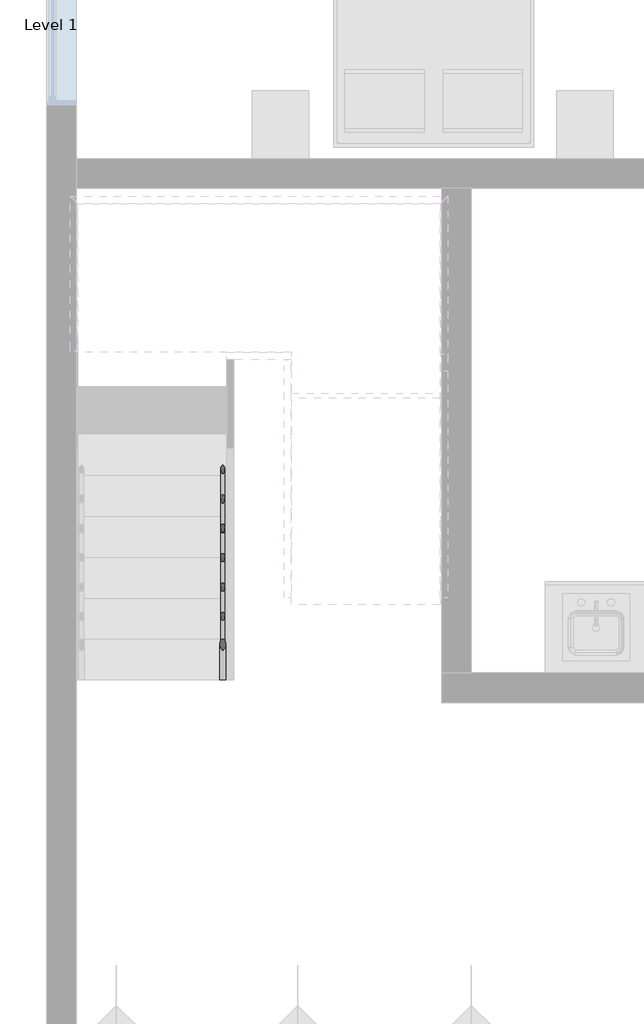
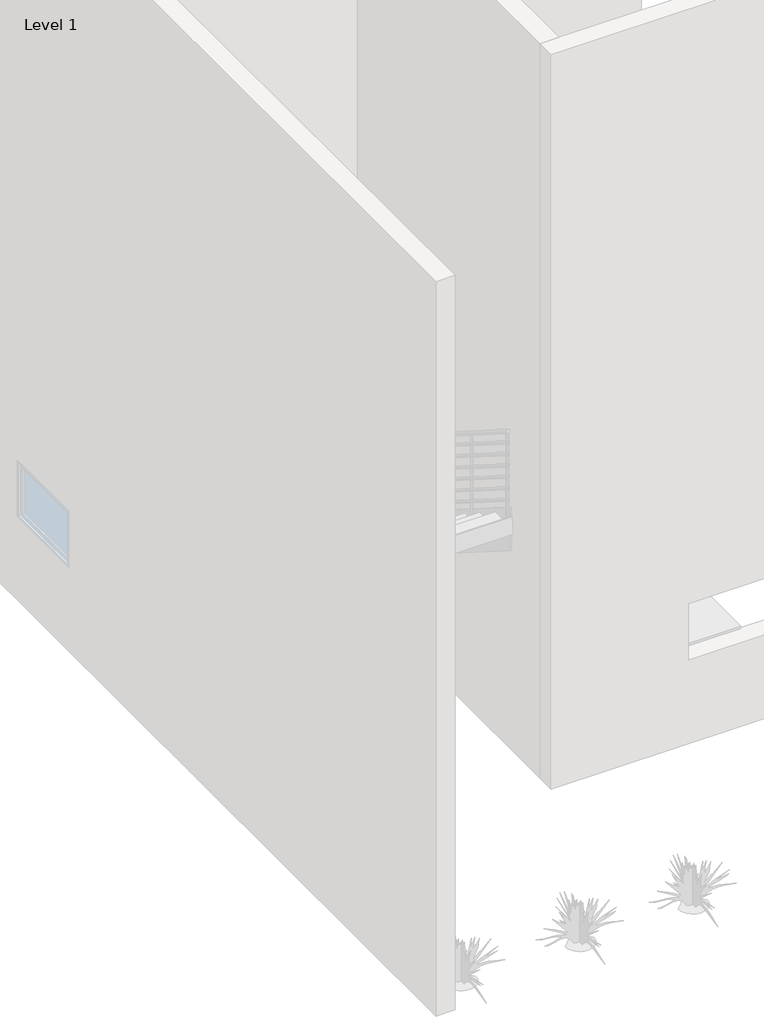
# One storey, part 2 of 4: 1 railing.
"""IFC4 building model written with IfcOpenShell, lengths in millimetres."""

from ifc_helpers import new_model, si_unit, point, frame, frame_2d, origin, place, context, project, spatial, circle_curve, ellipse_curve, trimmed, segment, composite_curve, outline, extrude, element, save
from ifc_brep_helpers import plane_surface, cylinder_surface, advanced_brep

model = new_model("IFC4")

# Units and contexts
model_context = context("Model", 3, world=origin())
ifc_project = project(units=[si_unit("LENGTHUNIT", "METRE", prefix="MILLI")], contexts=[model_context])

# Site, building, storey
site = spatial("IfcSite", under=ifc_project)
building = spatial("IfcBuilding", under=site)
storey = spatial("IfcBuildingStorey", under=building, Name="Level 1", Elevation=0.0)

# Railing
placement = place(None, origin())
element("IfcRailing", 1, ObjectType="900mm Pipe", at=placement, inside=storey, context=model_context, shape_type="SolidModel", body=[
    advanced_brep(
    [(-11027.5547869, 827.4280728, 1050.2491997), (-11067.5547869, 827.4280728, 1050.2491997), (-11027.5547869, 3046.614561, 2453.687295), (-11067.5547869, 3080.4214102, 2475.0671206)],
    [
        (0, 1, ellipse_curve(frame((-11047.5547869, 827.4280728, 1050.2491997), z_axis=(0.0, -1.0, 0.0), x_axis=(0.0, 0.0, -1.0)), 23.6638438, 20.0)),
        (1, 0, ellipse_curve(frame((-11047.5547869, 827.4280728, 1050.2491997), z_axis=(0.0, -1.0, 0.0), x_axis=(0.0, 0.0, -1.0)), 23.6638438, 20.0)),
        (2, 3, ellipse_curve(frame((-11047.5547869, 3063.5179856, 2464.3772078), z_axis=(0.7071067811865486, 0.5976263089853405, 0.37794549184843695), x_axis=(0.7071067811865465, -0.5976263089853425, -0.37794549184843734)), 28.2842712, 20.0)),
        (3, 2, ellipse_curve(frame((-11047.5547869, 3063.5179856, 2464.3772078), z_axis=(0.7071067811865486, 0.5976263089853405, 0.37794549184843695), x_axis=(0.7071067811865465, -0.5976263089853425, -0.37794549184843734)), 28.2842712, 20.0)),
        (0, 2),
        (3, 1),
    ],
    [
        plane_surface(frame((-11047.5547869, 827.4280728, 1073.9130435), z_axis=(0.0, -1.0, 0.0), x_axis=(0.0, 0.0, 1.0))),
        plane_surface(frame((-11047.5547869, 3052.8280728, 2481.2806324), z_axis=(0.7071067811865486, 0.5976263089853405, 0.37794549184843695), x_axis=(0.7071067811865466, -0.5976263089853422, -0.377945491848438))),
        cylinder_surface(frame((-11047.5547869, 838.1179856, 1057.0096189), z_axis=(0.0, -0.845171231398044, -0.5344956404098299), x_axis=(-1.0, 0.0, 0.0)), 20.0),
    ],
    [
        (0, [[1, 2]]),
        (1, [[3, 4]]),
        (2, [[-1, 5, -4, 6]]),
        (2, [[-2, -6, -3, -5]]),
    ],
),
    advanced_brep(
    [(-11019.9614494, 3032.8280728, 2445.2173913), (-11053.7682987, 3072.8280728, 2445.2173913), (-10566.3940799, 3032.8280728, 2445.2173913), (-10532.5872307, 3072.8280728, 2445.2173913)],
    [
        (0, 1, ellipse_curve(frame((-11036.8648741, 3052.8280728, 2445.2173913), z_axis=(-0.7071067811865486, -0.5976263089853405, -0.37794549184843695), x_axis=(-0.7071067811865466, 0.5976263089853426, 0.37794549184843723)), 28.2842712, 20.0)),
        (1, 0, ellipse_curve(frame((-11036.8648741, 3052.8280728, 2445.2173913), z_axis=(-0.7071067811865486, -0.5976263089853405, -0.37794549184843695), x_axis=(-0.7071067811865466, 0.5976263089853426, 0.37794549184843723)), 28.2842712, 20.0)),
        (2, 3, ellipse_curve(frame((-10549.4906553, 3052.8280728, 2445.2173913), z_axis=(0.7071067811865468, -0.5976263089853426, 0.3779454918484371), x_axis=(-0.7071067811865481, -0.5976263089853409, 0.3779454918484371)), 28.2842712, 20.0)),
        (3, 2, ellipse_curve(frame((-10549.4906553, 3052.8280728, 2445.2173913), z_axis=(0.7071067811865468, -0.5976263089853426, 0.3779454918484371), x_axis=(-0.7071067811865481, -0.5976263089853409, 0.3779454918484371)), 28.2842712, 20.0)),
        (0, 2),
        (3, 1),
    ],
    [
        plane_surface(frame((-11047.5547869, 3052.8280728, 2465.2173913), z_axis=(-0.7071067811865486, -0.5976263089853405, -0.37794549184843695), x_axis=(0.7071067811865466, -0.5976263089853422, -0.377945491848438))),
        plane_surface(frame((-10560.1805681, 3052.8280728, 2465.2173913), z_axis=(0.7071067811865467, -0.5976263089853425, 0.377945491848437), x_axis=(0.7071067811865482, 0.5976263089853412, -0.37794549184843623))),
        cylinder_surface(frame((-11047.5547869, 3052.8280728, 2445.2173913), z_axis=(-1.0, 0.0, 0.0), x_axis=(0.0, 1.0, 0.0)), 20.0),
    ],
    [
        (0, [[1, 2]]),
        (1, [[3, 4]]),
        (2, [[-1, 5, -4, 6]]),
        (2, [[-2, -6, -3, -5]]),
    ],
),
    advanced_brep(
    [(-10580.1805681, 2999.8347353, 2459.0038795), (-10540.1805681, 3033.6415846, 2437.6240539), (-10580.1805681, 1377.4280728, 3485.0318084), (-10540.1805681, 1377.4280728, 3485.0318084)],
    [
        (0, 1, ellipse_curve(frame((-10560.1805681, 3016.73816, 2448.3139667), z_axis=(-0.7071067811865468, 0.5976263089853426, -0.3779454918484371), x_axis=(0.7071067811865485, 0.5976263089853404, -0.3779454918484369)), 28.2842712, 20.0)),
        (1, 0, ellipse_curve(frame((-10560.1805681, 3016.73816, 2448.3139667), z_axis=(-0.7071067811865468, 0.5976263089853426, -0.3779454918484371), x_axis=(0.7071067811865485, 0.5976263089853404, -0.3779454918484369)), 28.2842712, 20.0)),
        (2, 3, ellipse_curve(frame((-10560.1805681, 1377.4280728, 3485.0318084), z_axis=(0.0, -1.0, 0.0), x_axis=(0.0, 0.0, -1.0)), 23.6638438, 20.0)),
        (3, 2, ellipse_curve(frame((-10560.1805681, 1377.4280728, 3485.0318084), z_axis=(0.0, -1.0, 0.0), x_axis=(0.0, 0.0, -1.0)), 23.6638438, 20.0)),
        (0, 2),
        (3, 1),
    ],
    [
        plane_surface(frame((-10560.1805681, 3027.4280728, 2465.2173913), z_axis=(-0.7071067811865467, 0.5976263089853425, -0.377945491848437), x_axis=(0.7071067811865482, 0.5976263089853412, -0.37794549184843623))),
        plane_surface(frame((-10560.1805681, 1377.4280728, 3508.6956522), z_axis=(0.0, -1.0, 0.0), x_axis=(0.0, 0.0, -1.0))),
        cylinder_surface(frame((-10560.1805681, 3016.73816, 2448.3139667), z_axis=(0.0, 0.845171231398044, -0.5344956404098297), x_axis=(1.0, 0.0, 0.0)), 20.0),
    ],
    [
        (0, [[1, 2]]),
        (1, [[3, 4]]),
        (2, [[-1, 5, -4, 6]]),
        (2, [[-2, -6, -3, -5]]),
    ],
),
    advanced_brep(
    [(-11062.5547869, 827.4280728, 931.1651606), (-11032.5547869, 827.4280728, 931.1651606), (-11062.5547869, 3031.7731625, 2325.2173913), (-11032.5547869, 3031.7731625, 2325.2173913), (-11062.5547869, 3067.8280728, 2325.2173913), (-11032.5547869, 3037.8280728, 2325.2173913), (-10545.1805681, 3067.8280728, 2325.2173913), (-10575.1805681, 3037.8280728, 2325.2173913), (-10545.1805681, 3023.082983, 2325.2173913), (-10575.1805681, 3023.082983, 2325.2173913), (-10545.1805681, 1377.4280728, 3365.9477693), (-10575.1805681, 1377.4280728, 3365.9477693)],
    [
        (0, 1, ellipse_curve(frame((-11047.5547869, 827.4280728, 931.1651606), z_axis=(0.0, -1.0, 0.0), x_axis=(0.0, 0.0, -1.0)), 17.7478828, 15.0)),
        (1, 0, ellipse_curve(frame((-11047.5547869, 827.4280728, 931.1651606), z_axis=(0.0, -1.0, 0.0), x_axis=(0.0, 0.0, -1.0)), 17.7478828, 15.0)),
        (0, 2),
        (2, 3, ellipse_curve(frame((-11047.5547869, 3031.7731625, 2325.2173913), z_axis=(0.0, -0.9605132043335073, -0.27823440531497545), x_axis=(0.0, 0.2782344053149749, -0.9605132043335074)), 15.6166515, 15.0)),
        (3, 1),
        (3, 2, ellipse_curve(frame((-11047.5547869, 3031.7731625, 2325.2173913), z_axis=(0.0, -0.9605132043335073, -0.27823440531497545), x_axis=(0.0, 0.2782344053149749, -0.9605132043335074)), 15.6166515, 15.0)),
        (2, 4),
        (4, 5, ellipse_curve(frame((-11047.5547869, 3052.8280728, 2325.2173913), z_axis=(-0.7071067811865487, -0.7071067811865464, 0.0), x_axis=(0.7071067811865464, -0.7071067811865486, 0.0)), 21.2132034, 15.0)),
        (5, 3),
        (5, 4, ellipse_curve(frame((-11047.5547869, 3052.8280728, 2325.2173913), z_axis=(-0.7071067811865487, -0.7071067811865464, 0.0), x_axis=(0.7071067811865464, -0.7071067811865486, 0.0)), 21.2132034, 15.0)),
        (4, 6),
        (6, 7, ellipse_curve(frame((-10560.1805681, 3052.8280728, 2325.2173913), z_axis=(-0.7071067811865464, 0.7071067811865487, 0.0), x_axis=(-0.7071067811865486, -0.7071067811865464, 0.0)), 21.2132034, 15.0)),
        (7, 5),
        (7, 6, ellipse_curve(frame((-10560.1805681, 3052.8280728, 2325.2173913), z_axis=(-0.7071067811865464, 0.7071067811865487, 0.0), x_axis=(-0.7071067811865486, -0.7071067811865464, 0.0)), 21.2132034, 15.0)),
        (6, 8),
        (8, 9, ellipse_curve(frame((-10560.1805681, 3023.082983, 2325.2173913), z_axis=(0.0, 0.9605132043335073, -0.27823440531497534), x_axis=(0.0, 0.2782344053149759, 0.9605132043335072)), 15.6166515, 15.0)),
        (9, 7),
        (9, 8, ellipse_curve(frame((-10560.1805681, 3023.082983, 2325.2173913), z_axis=(0.0, 0.9605132043335073, -0.27823440531497534), x_axis=(0.0, 0.2782344053149759, 0.9605132043335072)), 15.6166515, 15.0)),
        (10, 11, ellipse_curve(frame((-10560.1805681, 1377.4280728, 3365.9477693), z_axis=(0.0, -1.0, 0.0), x_axis=(0.0, 0.0, -1.0)), 17.7478828, 15.0)),
        (11, 10, ellipse_curve(frame((-10560.1805681, 1377.4280728, 3365.9477693), z_axis=(0.0, -1.0, 0.0), x_axis=(0.0, 0.0, -1.0)), 17.7478828, 15.0)),
        (8, 10),
        (11, 9),
    ],
    [
        plane_surface(frame((-11047.5547869, 827.4280728, 948.9130435), z_axis=(0.0, -1.0, 0.0), x_axis=(0.0, 0.0, 1.0))),
        cylinder_surface(frame((-11047.5547869, 835.4455074, 936.235475), z_axis=(0.0, -0.845171231398044, -0.5344956404098299), x_axis=(1.0, 0.0, 0.0)), 15.0),
        cylinder_surface(frame((-11047.5547869, 3027.4280728, 2325.2173913), z_axis=(0.0, -1.0, 0.0), x_axis=(1.0, 0.0, 0.0)), 15.0),
        cylinder_surface(frame((-11047.5547869, 3052.8280728, 2325.2173913), z_axis=(-1.0, 0.0, 0.0), x_axis=(0.0, -1.0, 0.0)), 15.0),
        cylinder_surface(frame((-10560.1805681, 3052.8280728, 2325.2173913), z_axis=(0.0, 1.0, 0.0), x_axis=(-1.0, 0.0, 0.0)), 15.0),
        plane_surface(frame((-10560.1805681, 1377.4280728, 3383.6956522), z_axis=(0.0, -1.0, 0.0), x_axis=(0.0, 0.0, -1.0))),
        cylinder_surface(frame((-10560.1805681, 3019.4106382, 2327.5398228), z_axis=(0.0, 0.8451712313980441, -0.5344956404098297), x_axis=(-1.0, 0.0, 0.0)), 15.0),
    ],
    [
        (0, [[1, 2]]),
        (1, [[-1, 3, 4, 5]]),
        (1, [[-2, -5, 6, -3]]),
        (2, [[-4, 7, 8, 9]]),
        (2, [[-6, -9, 10, -7]]),
        (3, [[-8, 11, 12, 13]]),
        (3, [[-10, -13, 14, -11]]),
        (4, [[-12, 15, 16, 17]]),
        (4, [[-14, -17, 18, -15]]),
        (5, [[19, 20]]),
        (6, [[-16, 21, -20, 22]]),
        (6, [[-18, -22, -19, -21]]),
    ],
),
    advanced_brep(
    [(-11062.5547869, 827.4280728, 806.1651606), (-11032.5547869, 827.4280728, 806.1651606), (-11062.5547869, 3031.7731625, 2200.2173913), (-11032.5547869, 3031.7731625, 2200.2173913), (-11062.5547869, 3067.8280728, 2200.2173913), (-11032.5547869, 3037.8280728, 2200.2173913), (-10545.1805681, 3067.8280728, 2200.2173913), (-10575.1805681, 3037.8280728, 2200.2173913), (-10545.1805681, 3023.082983, 2200.2173913), (-10575.1805681, 3023.082983, 2200.2173913), (-10545.1805681, 1377.4280728, 3240.9477693), (-10575.1805681, 1377.4280728, 3240.9477693)],
    [
        (0, 1, ellipse_curve(frame((-11047.5547869, 827.4280728, 806.1651606), z_axis=(0.0, -1.0, 0.0), x_axis=(0.0, 0.0, -1.0)), 17.7478828, 15.0)),
        (1, 0, ellipse_curve(frame((-11047.5547869, 827.4280728, 806.1651606), z_axis=(0.0, -1.0, 0.0), x_axis=(0.0, 0.0, -1.0)), 17.7478828, 15.0)),
        (0, 2),
        (2, 3, ellipse_curve(frame((-11047.5547869, 3031.7731625, 2200.2173913), z_axis=(0.0, -0.9605132043335073, -0.27823440531497545), x_axis=(0.0, 0.2782344053149749, -0.9605132043335074)), 15.6166515, 15.0)),
        (3, 1),
        (3, 2, ellipse_curve(frame((-11047.5547869, 3031.7731625, 2200.2173913), z_axis=(0.0, -0.9605132043335073, -0.27823440531497545), x_axis=(0.0, 0.2782344053149749, -0.9605132043335074)), 15.6166515, 15.0)),
        (2, 4),
        (4, 5, ellipse_curve(frame((-11047.5547869, 3052.8280728, 2200.2173913), z_axis=(-0.7071067811865487, -0.7071067811865464, 0.0), x_axis=(0.7071067811865464, -0.7071067811865486, 0.0)), 21.2132034, 15.0)),
        (5, 3),
        (5, 4, ellipse_curve(frame((-11047.5547869, 3052.8280728, 2200.2173913), z_axis=(-0.7071067811865487, -0.7071067811865464, 0.0), x_axis=(0.7071067811865464, -0.7071067811865486, 0.0)), 21.2132034, 15.0)),
        (4, 6),
        (6, 7, ellipse_curve(frame((-10560.1805681, 3052.8280728, 2200.2173913), z_axis=(-0.7071067811865464, 0.7071067811865487, 0.0), x_axis=(-0.7071067811865486, -0.7071067811865464, 0.0)), 21.2132034, 15.0)),
        (7, 5),
        (7, 6, ellipse_curve(frame((-10560.1805681, 3052.8280728, 2200.2173913), z_axis=(-0.7071067811865464, 0.7071067811865487, 0.0), x_axis=(-0.7071067811865486, -0.7071067811865464, 0.0)), 21.2132034, 15.0)),
        (6, 8),
        (8, 9, ellipse_curve(frame((-10560.1805681, 3023.082983, 2200.2173913), z_axis=(0.0, 0.9605132043335073, -0.27823440531497534), x_axis=(0.0, 0.2782344053149759, 0.9605132043335072)), 15.6166515, 15.0)),
        (9, 7),
        (9, 8, ellipse_curve(frame((-10560.1805681, 3023.082983, 2200.2173913), z_axis=(0.0, 0.9605132043335073, -0.27823440531497534), x_axis=(0.0, 0.2782344053149759, 0.9605132043335072)), 15.6166515, 15.0)),
        (10, 11, ellipse_curve(frame((-10560.1805681, 1377.4280728, 3240.9477693), z_axis=(0.0, -1.0, 0.0), x_axis=(0.0, 0.0, -1.0)), 17.7478828, 15.0)),
        (11, 10, ellipse_curve(frame((-10560.1805681, 1377.4280728, 3240.9477693), z_axis=(0.0, -1.0, 0.0), x_axis=(0.0, 0.0, -1.0)), 17.7478828, 15.0)),
        (8, 10),
        (11, 9),
    ],
    [
        plane_surface(frame((-11047.5547869, 827.4280728, 823.9130435), z_axis=(0.0, -1.0, 0.0), x_axis=(0.0, 0.0, 1.0))),
        cylinder_surface(frame((-11047.5547869, 835.4455074, 811.235475), z_axis=(0.0, -0.845171231398044, -0.5344956404098299), x_axis=(1.0, 0.0, 0.0)), 15.0),
        cylinder_surface(frame((-11047.5547869, 3027.4280728, 2200.2173913), z_axis=(0.0, -1.0, 0.0), x_axis=(1.0, 0.0, 0.0)), 15.0),
        cylinder_surface(frame((-11047.5547869, 3052.8280728, 2200.2173913), z_axis=(-1.0, 0.0, 0.0), x_axis=(0.0, -1.0, 0.0)), 15.0),
        cylinder_surface(frame((-10560.1805681, 3052.8280728, 2200.2173913), z_axis=(0.0, 1.0, 0.0), x_axis=(-1.0, 0.0, 0.0)), 15.0),
        plane_surface(frame((-10560.1805681, 1377.4280728, 3258.6956522), z_axis=(0.0, -1.0, 0.0), x_axis=(0.0, 0.0, -1.0))),
        cylinder_surface(frame((-10560.1805681, 3019.4106382, 2202.5398228), z_axis=(0.0, 0.845171231398044, -0.5344956404098297), x_axis=(-1.0, 0.0, 0.0)), 15.0),
    ],
    [
        (0, [[1, 2]]),
        (1, [[-1, 3, 4, 5]]),
        (1, [[-2, -5, 6, -3]]),
        (2, [[-4, 7, 8, 9]]),
        (2, [[-6, -9, 10, -7]]),
        (3, [[-8, 11, 12, 13]]),
        (3, [[-10, -13, 14, -11]]),
        (4, [[-12, 15, 16, 17]]),
        (4, [[-14, -17, 18, -15]]),
        (5, [[19, 20]]),
        (6, [[-16, 21, -20, 22]]),
        (6, [[-18, -22, -19, -21]]),
    ],
),
    advanced_brep(
    [(-11062.5547869, 827.4280728, 681.1651606), (-11032.5547869, 827.4280728, 681.1651606), (-11062.5547869, 3031.7731625, 2075.2173913), (-11032.5547869, 3031.7731625, 2075.2173913), (-11062.5547869, 3067.8280728, 2075.2173913), (-11032.5547869, 3037.8280728, 2075.2173913), (-10545.1805681, 3067.8280728, 2075.2173913), (-10575.1805681, 3037.8280728, 2075.2173913), (-10545.1805681, 3023.082983, 2075.2173913), (-10575.1805681, 3023.082983, 2075.2173913), (-10545.1805681, 1377.4280728, 3115.9477693), (-10575.1805681, 1377.4280728, 3115.9477693)],
    [
        (0, 1, ellipse_curve(frame((-11047.5547869, 827.4280728, 681.1651606), z_axis=(0.0, -1.0, 0.0), x_axis=(0.0, 0.0, -1.0)), 17.7478828, 15.0)),
        (1, 0, ellipse_curve(frame((-11047.5547869, 827.4280728, 681.1651606), z_axis=(0.0, -1.0, 0.0), x_axis=(0.0, 0.0, -1.0)), 17.7478828, 15.0)),
        (0, 2),
        (2, 3, ellipse_curve(frame((-11047.5547869, 3031.7731625, 2075.2173913), z_axis=(0.0, -0.9605132043335073, -0.27823440531497545), x_axis=(0.0, 0.2782344053149749, -0.9605132043335074)), 15.6166515, 15.0)),
        (3, 1),
        (3, 2, ellipse_curve(frame((-11047.5547869, 3031.7731625, 2075.2173913), z_axis=(0.0, -0.9605132043335073, -0.27823440531497545), x_axis=(0.0, 0.2782344053149749, -0.9605132043335074)), 15.6166515, 15.0)),
        (2, 4),
        (4, 5, ellipse_curve(frame((-11047.5547869, 3052.8280728, 2075.2173913), z_axis=(-0.7071067811865487, -0.7071067811865464, 0.0), x_axis=(0.7071067811865464, -0.7071067811865486, 0.0)), 21.2132034, 15.0)),
        (5, 3),
        (5, 4, ellipse_curve(frame((-11047.5547869, 3052.8280728, 2075.2173913), z_axis=(-0.7071067811865487, -0.7071067811865464, 0.0), x_axis=(0.7071067811865464, -0.7071067811865486, 0.0)), 21.2132034, 15.0)),
        (4, 6),
        (6, 7, ellipse_curve(frame((-10560.1805681, 3052.8280728, 2075.2173913), z_axis=(-0.7071067811865464, 0.7071067811865487, 0.0), x_axis=(-0.7071067811865486, -0.7071067811865464, 0.0)), 21.2132034, 15.0)),
        (7, 5),
        (7, 6, ellipse_curve(frame((-10560.1805681, 3052.8280728, 2075.2173913), z_axis=(-0.7071067811865464, 0.7071067811865487, 0.0), x_axis=(-0.7071067811865486, -0.7071067811865464, 0.0)), 21.2132034, 15.0)),
        (6, 8),
        (8, 9, ellipse_curve(frame((-10560.1805681, 3023.082983, 2075.2173913), z_axis=(0.0, 0.9605132043335073, -0.2782344053149754), x_axis=(0.0, 0.27823440531497584, 0.9605132043335073)), 15.6166515, 15.0)),
        (9, 7),
        (9, 8, ellipse_curve(frame((-10560.1805681, 3023.082983, 2075.2173913), z_axis=(0.0, 0.9605132043335073, -0.2782344053149754), x_axis=(0.0, 0.27823440531497584, 0.9605132043335073)), 15.6166515, 15.0)),
        (10, 11, ellipse_curve(frame((-10560.1805681, 1377.4280728, 3115.9477693), z_axis=(0.0, -1.0, 0.0), x_axis=(0.0, 0.0, -1.0)), 17.7478828, 15.0)),
        (11, 10, ellipse_curve(frame((-10560.1805681, 1377.4280728, 3115.9477693), z_axis=(0.0, -1.0, 0.0), x_axis=(0.0, 0.0, -1.0)), 17.7478828, 15.0)),
        (8, 10),
        (11, 9),
    ],
    [
        plane_surface(frame((-11047.5547869, 827.4280728, 698.9130435), z_axis=(0.0, -1.0, 0.0), x_axis=(0.0, 0.0, 1.0))),
        cylinder_surface(frame((-11047.5547869, 835.4455074, 686.235475), z_axis=(0.0, -0.845171231398044, -0.5344956404098299), x_axis=(1.0, 0.0, 0.0)), 15.0),
        cylinder_surface(frame((-11047.5547869, 3027.4280728, 2075.2173913), z_axis=(0.0, -1.0, 0.0), x_axis=(1.0, 0.0, 0.0)), 15.0),
        cylinder_surface(frame((-11047.5547869, 3052.8280728, 2075.2173913), z_axis=(-1.0, 0.0, 0.0), x_axis=(0.0, -1.0, 0.0)), 15.0),
        cylinder_surface(frame((-10560.1805681, 3052.8280728, 2075.2173913), z_axis=(0.0, 1.0, 0.0), x_axis=(-1.0, 0.0, 0.0)), 15.0),
        plane_surface(frame((-10560.1805681, 1377.4280728, 3133.6956522), z_axis=(0.0, -1.0, 0.0), x_axis=(0.0, 0.0, -1.0))),
        cylinder_surface(frame((-10560.1805681, 3019.4106382, 2077.5398228), z_axis=(0.0, 0.845171231398044, -0.5344956404098298), x_axis=(-1.0, 0.0, 0.0)), 15.0),
    ],
    [
        (0, [[1, 2]]),
        (1, [[-1, 3, 4, 5]]),
        (1, [[-2, -5, 6, -3]]),
        (2, [[-4, 7, 8, 9]]),
        (2, [[-6, -9, 10, -7]]),
        (3, [[-8, 11, 12, 13]]),
        (3, [[-10, -13, 14, -11]]),
        (4, [[-12, 15, 16, 17]]),
        (4, [[-14, -17, 18, -15]]),
        (5, [[19, 20]]),
        (6, [[-16, 21, -20, 22]]),
        (6, [[-18, -22, -19, -21]]),
    ],
),
    advanced_brep(
    [(-11062.5547869, 827.4280728, 556.1651606), (-11032.5547869, 827.4280728, 556.1651606), (-11062.5547869, 3031.7731625, 1950.2173913), (-11032.5547869, 3031.7731625, 1950.2173913), (-11062.5547869, 3067.8280728, 1950.2173913), (-11032.5547869, 3037.8280728, 1950.2173913), (-10545.1805681, 3067.8280728, 1950.2173913), (-10575.1805681, 3037.8280728, 1950.2173913), (-10545.1805681, 3023.082983, 1950.2173913), (-10575.1805681, 3023.082983, 1950.2173913), (-10545.1805681, 1377.4280728, 2990.9477693), (-10575.1805681, 1377.4280728, 2990.9477693)],
    [
        (0, 1, ellipse_curve(frame((-11047.5547869, 827.4280728, 556.1651606), z_axis=(0.0, -1.0, 0.0), x_axis=(0.0, 0.0, -1.0)), 17.7478828, 15.0)),
        (1, 0, ellipse_curve(frame((-11047.5547869, 827.4280728, 556.1651606), z_axis=(0.0, -1.0, 0.0), x_axis=(0.0, 0.0, -1.0)), 17.7478828, 15.0)),
        (0, 2),
        (2, 3, ellipse_curve(frame((-11047.5547869, 3031.7731625, 1950.2173913), z_axis=(0.0, -0.9605132043335073, -0.27823440531497545), x_axis=(0.0, 0.2782344053149749, -0.9605132043335074)), 15.6166515, 15.0)),
        (3, 1),
        (3, 2, ellipse_curve(frame((-11047.5547869, 3031.7731625, 1950.2173913), z_axis=(0.0, -0.9605132043335073, -0.27823440531497545), x_axis=(0.0, 0.2782344053149749, -0.9605132043335074)), 15.6166515, 15.0)),
        (2, 4),
        (4, 5, ellipse_curve(frame((-11047.5547869, 3052.8280728, 1950.2173913), z_axis=(-0.7071067811865487, -0.7071067811865464, 0.0), x_axis=(0.7071067811865464, -0.7071067811865486, 0.0)), 21.2132034, 15.0)),
        (5, 3),
        (5, 4, ellipse_curve(frame((-11047.5547869, 3052.8280728, 1950.2173913), z_axis=(-0.7071067811865487, -0.7071067811865464, 0.0), x_axis=(0.7071067811865464, -0.7071067811865486, 0.0)), 21.2132034, 15.0)),
        (4, 6),
        (6, 7, ellipse_curve(frame((-10560.1805681, 3052.8280728, 1950.2173913), z_axis=(-0.7071067811865464, 0.7071067811865487, 0.0), x_axis=(-0.7071067811865486, -0.7071067811865464, 0.0)), 21.2132034, 15.0)),
        (7, 5),
        (7, 6, ellipse_curve(frame((-10560.1805681, 3052.8280728, 1950.2173913), z_axis=(-0.7071067811865464, 0.7071067811865487, 0.0), x_axis=(-0.7071067811865486, -0.7071067811865464, 0.0)), 21.2132034, 15.0)),
        (6, 8),
        (8, 9, ellipse_curve(frame((-10560.1805681, 3023.082983, 1950.2173913), z_axis=(0.0, 0.9605132043335073, -0.27823440531497534), x_axis=(0.0, 0.2782344053149759, 0.9605132043335072)), 15.6166515, 15.0)),
        (9, 7),
        (9, 8, ellipse_curve(frame((-10560.1805681, 3023.082983, 1950.2173913), z_axis=(0.0, 0.9605132043335073, -0.27823440531497534), x_axis=(0.0, 0.2782344053149759, 0.9605132043335072)), 15.6166515, 15.0)),
        (10, 11, ellipse_curve(frame((-10560.1805681, 1377.4280728, 2990.9477693), z_axis=(0.0, -1.0, 0.0), x_axis=(0.0, 0.0, -1.0)), 17.7478828, 15.0)),
        (11, 10, ellipse_curve(frame((-10560.1805681, 1377.4280728, 2990.9477693), z_axis=(0.0, -1.0, 0.0), x_axis=(0.0, 0.0, -1.0)), 17.7478828, 15.0)),
        (8, 10),
        (11, 9),
    ],
    [
        plane_surface(frame((-11047.5547869, 827.4280728, 573.9130435), z_axis=(0.0, -1.0, 0.0), x_axis=(0.0, 0.0, 1.0))),
        cylinder_surface(frame((-11047.5547869, 835.4455074, 561.235475), z_axis=(0.0, -0.845171231398044, -0.5344956404098299), x_axis=(1.0, 0.0, 0.0)), 15.0),
        cylinder_surface(frame((-11047.5547869, 3027.4280728, 1950.2173913), z_axis=(0.0, -1.0, 0.0), x_axis=(1.0, 0.0, 0.0)), 15.0),
        cylinder_surface(frame((-11047.5547869, 3052.8280728, 1950.2173913), z_axis=(-1.0, 0.0, 0.0), x_axis=(0.0, -1.0, 0.0)), 15.0),
        cylinder_surface(frame((-10560.1805681, 3052.8280728, 1950.2173913), z_axis=(0.0, 1.0, 0.0), x_axis=(-1.0, 0.0, 0.0)), 15.0),
        plane_surface(frame((-10560.1805681, 1377.4280728, 3008.6956522), z_axis=(0.0, -1.0, 0.0), x_axis=(0.0, 0.0, -1.0))),
        cylinder_surface(frame((-10560.1805681, 3019.4106382, 1952.5398228), z_axis=(0.0, 0.845171231398044, -0.5344956404098297), x_axis=(-1.0, 0.0, 0.0)), 15.0),
    ],
    [
        (0, [[1, 2]]),
        (1, [[-1, 3, 4, 5]]),
        (1, [[-2, -5, 6, -3]]),
        (2, [[-4, 7, 8, 9]]),
        (2, [[-6, -9, 10, -7]]),
        (3, [[-8, 11, 12, 13]]),
        (3, [[-10, -13, 14, -11]]),
        (4, [[-12, 15, 16, 17]]),
        (4, [[-14, -17, 18, -15]]),
        (5, [[19, 20]]),
        (6, [[-16, 21, -20, 22]]),
        (6, [[-18, -22, -19, -21]]),
    ],
),
    advanced_brep(
    [(-11062.5547869, 827.4280728, 431.1651606), (-11032.5547869, 827.4280728, 431.1651606), (-11062.5547869, 3031.7731625, 1825.2173913), (-11032.5547869, 3031.7731625, 1825.2173913), (-11062.5547869, 3067.8280728, 1825.2173913), (-11032.5547869, 3037.8280728, 1825.2173913), (-10545.1805681, 3067.8280728, 1825.2173913), (-10575.1805681, 3037.8280728, 1825.2173913), (-10545.1805681, 3023.082983, 1825.2173913), (-10575.1805681, 3023.082983, 1825.2173913), (-10545.1805681, 1377.4280728, 2865.9477693), (-10575.1805681, 1377.4280728, 2865.9477693)],
    [
        (0, 1, ellipse_curve(frame((-11047.5547869, 827.4280728, 431.1651606), z_axis=(0.0, -1.0, 0.0), x_axis=(0.0, 0.0, -1.0)), 17.7478828, 15.0)),
        (1, 0, ellipse_curve(frame((-11047.5547869, 827.4280728, 431.1651606), z_axis=(0.0, -1.0, 0.0), x_axis=(0.0, 0.0, -1.0)), 17.7478828, 15.0)),
        (0, 2),
        (2, 3, ellipse_curve(frame((-11047.5547869, 3031.7731625, 1825.2173913), z_axis=(0.0, -0.9605132043335073, -0.27823440531497545), x_axis=(0.0, 0.2782344053149749, -0.9605132043335074)), 15.6166515, 15.0)),
        (3, 1),
        (3, 2, ellipse_curve(frame((-11047.5547869, 3031.7731625, 1825.2173913), z_axis=(0.0, -0.9605132043335073, -0.27823440531497545), x_axis=(0.0, 0.2782344053149749, -0.9605132043335074)), 15.6166515, 15.0)),
        (2, 4),
        (4, 5, ellipse_curve(frame((-11047.5547869, 3052.8280728, 1825.2173913), z_axis=(-0.7071067811865487, -0.7071067811865464, 0.0), x_axis=(0.7071067811865464, -0.7071067811865486, 0.0)), 21.2132034, 15.0)),
        (5, 3),
        (5, 4, ellipse_curve(frame((-11047.5547869, 3052.8280728, 1825.2173913), z_axis=(-0.7071067811865487, -0.7071067811865464, 0.0), x_axis=(0.7071067811865464, -0.7071067811865486, 0.0)), 21.2132034, 15.0)),
        (4, 6),
        (6, 7, ellipse_curve(frame((-10560.1805681, 3052.8280728, 1825.2173913), z_axis=(-0.7071067811865464, 0.7071067811865487, 0.0), x_axis=(-0.7071067811865486, -0.7071067811865464, 0.0)), 21.2132034, 15.0)),
        (7, 5),
        (7, 6, ellipse_curve(frame((-10560.1805681, 3052.8280728, 1825.2173913), z_axis=(-0.7071067811865464, 0.7071067811865487, 0.0), x_axis=(-0.7071067811865486, -0.7071067811865464, 0.0)), 21.2132034, 15.0)),
        (6, 8),
        (8, 9, ellipse_curve(frame((-10560.1805681, 3023.082983, 1825.2173913), z_axis=(0.0, 0.9605132043335073, -0.27823440531497534), x_axis=(0.0, 0.2782344053149759, 0.9605132043335072)), 15.6166515, 15.0)),
        (9, 7),
        (9, 8, ellipse_curve(frame((-10560.1805681, 3023.082983, 1825.2173913), z_axis=(0.0, 0.9605132043335073, -0.27823440531497534), x_axis=(0.0, 0.2782344053149759, 0.9605132043335072)), 15.6166515, 15.0)),
        (10, 11, ellipse_curve(frame((-10560.1805681, 1377.4280728, 2865.9477693), z_axis=(0.0, -1.0, 0.0), x_axis=(0.0, 0.0, -1.0)), 17.7478828, 15.0)),
        (11, 10, ellipse_curve(frame((-10560.1805681, 1377.4280728, 2865.9477693), z_axis=(0.0, -1.0, 0.0), x_axis=(0.0, 0.0, -1.0)), 17.7478828, 15.0)),
        (8, 10),
        (11, 9),
    ],
    [
        plane_surface(frame((-11047.5547869, 827.4280728, 448.9130435), z_axis=(0.0, -1.0, 0.0), x_axis=(0.0, 0.0, 1.0))),
        cylinder_surface(frame((-11047.5547869, 835.4455074, 436.235475), z_axis=(0.0, -0.845171231398044, -0.5344956404098299), x_axis=(1.0, 0.0, 0.0)), 15.0),
        cylinder_surface(frame((-11047.5547869, 3027.4280728, 1825.2173913), z_axis=(0.0, -1.0, 0.0), x_axis=(1.0, 0.0, 0.0)), 15.0),
        cylinder_surface(frame((-11047.5547869, 3052.8280728, 1825.2173913), z_axis=(-1.0, 0.0, 0.0), x_axis=(0.0, -1.0, 0.0)), 15.0),
        cylinder_surface(frame((-10560.1805681, 3052.8280728, 1825.2173913), z_axis=(0.0, 1.0, 0.0), x_axis=(-1.0, 0.0, 0.0)), 15.0),
        plane_surface(frame((-10560.1805681, 1377.4280728, 2883.6956522), z_axis=(0.0, -1.0, 0.0), x_axis=(0.0, 0.0, -1.0))),
        cylinder_surface(frame((-10560.1805681, 3019.4106382, 1827.5398228), z_axis=(0.0, 0.8451712313980441, -0.5344956404098297), x_axis=(-1.0, 0.0, 0.0)), 15.0),
    ],
    [
        (0, [[1, 2]]),
        (1, [[-1, 3, 4, 5]]),
        (1, [[-2, -5, 6, -3]]),
        (2, [[-4, 7, 8, 9]]),
        (2, [[-6, -9, 10, -7]]),
        (3, [[-8, 11, 12, 13]]),
        (3, [[-10, -13, 14, -11]]),
        (4, [[-12, 15, 16, 17]]),
        (4, [[-14, -17, 18, -15]]),
        (5, [[19, 20]]),
        (6, [[-16, 21, -20, 22]]),
        (6, [[-18, -22, -19, -21]]),
    ],
),
    advanced_brep(
    [(-11062.5547869, 827.4280728, 306.1651606), (-11032.5547869, 827.4280728, 306.1651606), (-11062.5547869, 3031.7731625, 1700.2173913), (-11032.5547869, 3031.7731625, 1700.2173913), (-11062.5547869, 3067.8280728, 1700.2173913), (-11032.5547869, 3037.8280728, 1700.2173913), (-10545.1805681, 3067.8280728, 1700.2173913), (-10575.1805681, 3037.8280728, 1700.2173913), (-10545.1805681, 3023.082983, 1700.2173913), (-10575.1805681, 3023.082983, 1700.2173913), (-10545.1805681, 1377.4280728, 2740.9477693), (-10575.1805681, 1377.4280728, 2740.9477693)],
    [
        (0, 1, ellipse_curve(frame((-11047.5547869, 827.4280728, 306.1651606), z_axis=(0.0, -1.0, 0.0), x_axis=(0.0, 0.0, -1.0)), 17.7478828, 15.0)),
        (1, 0, ellipse_curve(frame((-11047.5547869, 827.4280728, 306.1651606), z_axis=(0.0, -1.0, 0.0), x_axis=(0.0, 0.0, -1.0)), 17.7478828, 15.0)),
        (0, 2),
        (2, 3, ellipse_curve(frame((-11047.5547869, 3031.7731625, 1700.2173913), z_axis=(0.0, -0.9605132043335073, -0.27823440531497545), x_axis=(0.0, 0.2782344053149749, -0.9605132043335074)), 15.6166515, 15.0)),
        (3, 1),
        (3, 2, ellipse_curve(frame((-11047.5547869, 3031.7731625, 1700.2173913), z_axis=(0.0, -0.9605132043335073, -0.27823440531497545), x_axis=(0.0, 0.2782344053149749, -0.9605132043335074)), 15.6166515, 15.0)),
        (2, 4),
        (4, 5, ellipse_curve(frame((-11047.5547869, 3052.8280728, 1700.2173913), z_axis=(-0.7071067811865487, -0.7071067811865464, 0.0), x_axis=(0.7071067811865464, -0.7071067811865486, 0.0)), 21.2132034, 15.0)),
        (5, 3),
        (5, 4, ellipse_curve(frame((-11047.5547869, 3052.8280728, 1700.2173913), z_axis=(-0.7071067811865487, -0.7071067811865464, 0.0), x_axis=(0.7071067811865464, -0.7071067811865486, 0.0)), 21.2132034, 15.0)),
        (4, 6),
        (6, 7, ellipse_curve(frame((-10560.1805681, 3052.8280728, 1700.2173913), z_axis=(-0.7071067811865464, 0.7071067811865487, 0.0), x_axis=(-0.7071067811865486, -0.7071067811865464, 0.0)), 21.2132034, 15.0)),
        (7, 5),
        (7, 6, ellipse_curve(frame((-10560.1805681, 3052.8280728, 1700.2173913), z_axis=(-0.7071067811865464, 0.7071067811865487, 0.0), x_axis=(-0.7071067811865486, -0.7071067811865464, 0.0)), 21.2132034, 15.0)),
        (6, 8),
        (8, 9, ellipse_curve(frame((-10560.1805681, 3023.082983, 1700.2173913), z_axis=(0.0, 0.9605132043335073, -0.27823440531497534), x_axis=(0.0, 0.2782344053149759, 0.9605132043335072)), 15.6166515, 15.0)),
        (9, 7),
        (9, 8, ellipse_curve(frame((-10560.1805681, 3023.082983, 1700.2173913), z_axis=(0.0, 0.9605132043335073, -0.27823440531497534), x_axis=(0.0, 0.2782344053149759, 0.9605132043335072)), 15.6166515, 15.0)),
        (10, 11, ellipse_curve(frame((-10560.1805681, 1377.4280728, 2740.9477693), z_axis=(0.0, -1.0, 0.0), x_axis=(0.0, 0.0, -1.0)), 17.7478828, 15.0)),
        (11, 10, ellipse_curve(frame((-10560.1805681, 1377.4280728, 2740.9477693), z_axis=(0.0, -1.0, 0.0), x_axis=(0.0, 0.0, -1.0)), 17.7478828, 15.0)),
        (8, 10),
        (11, 9),
    ],
    [
        plane_surface(frame((-11047.5547869, 827.4280728, 323.9130435), z_axis=(0.0, -1.0, 0.0), x_axis=(0.0, 0.0, 1.0))),
        cylinder_surface(frame((-11047.5547869, 835.4455074, 311.235475), z_axis=(0.0, -0.845171231398044, -0.5344956404098299), x_axis=(1.0, 0.0, 0.0)), 15.0),
        cylinder_surface(frame((-11047.5547869, 3027.4280728, 1700.2173913), z_axis=(0.0, -1.0, 0.0), x_axis=(1.0, 0.0, 0.0)), 15.0),
        cylinder_surface(frame((-11047.5547869, 3052.8280728, 1700.2173913), z_axis=(-1.0, 0.0, 0.0), x_axis=(0.0, -1.0, 0.0)), 15.0),
        cylinder_surface(frame((-10560.1805681, 3052.8280728, 1700.2173913), z_axis=(0.0, 1.0, 0.0), x_axis=(-1.0, 0.0, 0.0)), 15.0),
        plane_surface(frame((-10560.1805681, 1377.4280728, 2758.6956522), z_axis=(0.0, -1.0, 0.0), x_axis=(0.0, 0.0, -1.0))),
        cylinder_surface(frame((-10560.1805681, 3019.4106382, 1702.5398228), z_axis=(0.0, 0.845171231398044, -0.5344956404098297), x_axis=(-1.0, 0.0, 0.0)), 15.0),
    ],
    [
        (0, [[1, 2]]),
        (1, [[-1, 3, 4, 5]]),
        (1, [[-2, -5, 6, -3]]),
        (2, [[-4, 7, 8, 9]]),
        (2, [[-6, -9, 10, -7]]),
        (3, [[-8, 11, 12, 13]]),
        (3, [[-10, -13, 14, -11]]),
        (4, [[-12, 15, 16, 17]]),
        (4, [[-14, -17, 18, -15]]),
        (5, [[19, 20]]),
        (6, [[-16, 21, -20, 22]]),
        (6, [[-18, -22, -19, -21]]),
    ],
),
    advanced_brep(
    [(-10572.6805681, 2027.4280728, 3050.3007709), (-10572.6805681, 2027.4280728, 2086.9565217), (-10547.6805681, 2027.4280728, 2086.9565217), (-10547.6805681, 2027.4280728, 3050.3007709)],
    [
        (0, 1),
        (1, 2, circle_curve(frame((-10560.1805681, 2027.4280728, 2086.9565217), z_axis=(0.0, 0.0, 1.0), x_axis=(1.0, 0.0, 0.0)), 12.5)),
        (2, 3),
        (3, 0, ellipse_curve(frame((-10560.1805681, 2027.4280728, 3050.3007709), z_axis=(0.0, -0.5344956404098286, -0.8451712313980447), x_axis=(0.0, -0.8451712313980447, 0.5344956404098286)), 14.7899024, 12.5)),
        (0, 3, ellipse_curve(frame((-10560.1805681, 2027.4280728, 3050.3007709), z_axis=(0.0, -0.5344956404098286, -0.8451712313980447), x_axis=(0.0, -0.8451712313980447, 0.5344956404098286)), 14.7899024, 12.5)),
        (2, 1, circle_curve(frame((-10560.1805681, 2027.4280728, 2086.9565217), z_axis=(0.0, 0.0, 1.0), x_axis=(1.0, 0.0, 0.0)), 12.5)),
    ],
    [
        cylinder_surface(frame((-10560.1805681, 2027.4280728, 1986.9565217), z_axis=(0.0, 0.0, 1.0), x_axis=(1.0, 0.0, 0.0)), 12.5),
        plane_surface(frame((-10535.1805681, 2002.4280728, 3066.1110476), z_axis=(0.0, 0.5344956404098286, 0.8451712313980447), x_axis=(-1.0, 0.0, 0.0))),
        plane_surface(frame((-10535.1805681, 2052.4280728, 2086.9565217), z_axis=(0.0, 0.0, -1.0), x_axis=(-1.0, 0.0, 0.0))),
    ],
    [
        (0, [[1, 2, 3, 4]]),
        (0, [[-1, 5, -3, 6]]),
        (1, [[-4, -5]]),
        (2, [[-2, -6]]),
    ],
),
    advanced_brep(
    [(-11035.0547869, 2827.4280728, 2291.4074903), (-11035.0547869, 2827.4280728, 1391.3043478), (-11060.0547869, 2827.4280728, 1391.3043478), (-11060.0547869, 2827.4280728, 2291.4074903)],
    [
        (0, 1),
        (1, 2, circle_curve(frame((-11047.5547869, 2827.4280728, 1391.3043478), z_axis=(0.0, 0.0, 1.0), x_axis=(-1.0, 0.0, 0.0)), 12.5)),
        (2, 3),
        (3, 0, ellipse_curve(frame((-11047.5547869, 2827.4280728, 2291.4074903), z_axis=(0.0, 0.5344956404098302, -0.8451712313980437), x_axis=(0.0, 0.8451712313980437, 0.53449564040983)), 14.7899024, 12.5)),
        (0, 3, ellipse_curve(frame((-11047.5547869, 2827.4280728, 2291.4074903), z_axis=(0.0, 0.5344956404098302, -0.8451712313980437), x_axis=(0.0, 0.8451712313980437, 0.53449564040983)), 14.7899024, 12.5)),
        (2, 1, circle_curve(frame((-11047.5547869, 2827.4280728, 1391.3043478), z_axis=(0.0, 0.0, 1.0), x_axis=(-1.0, 0.0, 0.0)), 12.5)),
    ],
    [
        cylinder_surface(frame((-11047.5547869, 2827.4280728, 1291.3043478), z_axis=(0.0, 0.0, 1.0), x_axis=(-1.0, 0.0, 0.0)), 12.5),
        plane_surface(frame((-11072.5547869, 2852.4280728, 2307.217767), z_axis=(0.0, -0.5344956404098302, 0.8451712313980437), x_axis=(1.0, 0.0, 0.0))),
        plane_surface(frame((-11072.5547869, 2802.4280728, 1391.3043478), z_axis=(0.0, 0.0, -1.0), x_axis=(1.0, 0.0, 0.0))),
    ],
    [
        (0, [[1, 2, 3, 4]]),
        (0, [[-1, 5, -3, 6]]),
        (1, [[-4, -5]]),
        (2, [[-2, -6]]),
    ],
),
    advanced_brep(
    [(-11035.0547869, 1827.4280728, 1658.9964231), (-11035.0547869, 1827.4280728, 695.6521739), (-11060.0547869, 1827.4280728, 695.6521739), (-11060.0547869, 1827.4280728, 1658.9964231)],
    [
        (0, 1),
        (1, 2, circle_curve(frame((-11047.5547869, 1827.4280728, 695.6521739), z_axis=(0.0, 0.0, 1.0), x_axis=(-1.0, 0.0, 0.0)), 12.5)),
        (2, 3),
        (3, 0, ellipse_curve(frame((-11047.5547869, 1827.4280728, 1658.9964231), z_axis=(0.0, 0.5344956404098286, -0.8451712313980447), x_axis=(0.0, 0.8451712313980447, 0.5344956404098286)), 14.7899024, 12.5)),
        (0, 3, ellipse_curve(frame((-11047.5547869, 1827.4280728, 1658.9964231), z_axis=(0.0, 0.5344956404098286, -0.8451712313980447), x_axis=(0.0, 0.8451712313980447, 0.5344956404098286)), 14.7899024, 12.5)),
        (2, 1, circle_curve(frame((-11047.5547869, 1827.4280728, 695.6521739), z_axis=(0.0, 0.0, 1.0), x_axis=(-1.0, 0.0, 0.0)), 12.5)),
    ],
    [
        cylinder_surface(frame((-11047.5547869, 1827.4280728, 595.6521739), z_axis=(0.0, 0.0, 1.0), x_axis=(-1.0, 0.0, 0.0)), 12.5),
        plane_surface(frame((-11072.5547869, 1852.4280728, 1674.8066998), z_axis=(0.0, -0.5344956404098286, 0.8451712313980447), x_axis=(1.0, 0.0, 0.0))),
        plane_surface(frame((-11072.5547869, 1802.4280728, 695.6521739), z_axis=(0.0, 0.0, -1.0), x_axis=(1.0, 0.0, 0.0))),
    ],
    [
        (0, [[1, 2, 3, 4]]),
        (0, [[-1, 5, -3, 6]]),
        (1, [[-4, -5]]),
        (2, [[-2, -6]]),
    ],
),
    advanced_brep(
    [(-10572.6805681, 3027.4280728, 2417.8897037), (-10572.6805681, 3027.4280728, 1565.2173913), (-10547.6805681, 3027.4280728, 1565.2173913), (-10547.6805681, 3027.4280728, 2417.8897037)],
    [
        (0, 1),
        (1, 2, circle_curve(frame((-10560.1805681, 3027.4280728, 1565.2173913), z_axis=(0.0, 0.0, 1.0), x_axis=(1.0, 0.0, 0.0)), 12.5)),
        (2, 3),
        (3, 0, ellipse_curve(frame((-10560.1805681, 3027.4280728, 2417.8897037), z_axis=(0.0, -0.5344956404098302, -0.8451712313980437), x_axis=(0.0, -0.8451712313980437, 0.53449564040983)), 14.7899024, 12.5)),
        (0, 3, ellipse_curve(frame((-10560.1805681, 3027.4280728, 2417.8897037), z_axis=(0.0, -0.5344956404098302, -0.8451712313980437), x_axis=(0.0, -0.8451712313980437, 0.53449564040983)), 14.7899024, 12.5)),
        (2, 1, circle_curve(frame((-10560.1805681, 3027.4280728, 1565.2173913), z_axis=(0.0, 0.0, 1.0), x_axis=(1.0, 0.0, 0.0)), 12.5)),
    ],
    [
        cylinder_surface(frame((-10560.1805681, 3027.4280728, 1465.2173913), z_axis=(0.0, 0.0, 1.0), x_axis=(1.0, 0.0, 0.0)), 12.5),
        plane_surface(frame((-10535.1805681, 3002.4280728, 2433.6999804), z_axis=(0.0, 0.5344956404098302, 0.8451712313980437), x_axis=(-1.0, 0.0, 0.0))),
        plane_surface(frame((-10535.1805681, 3052.4280728, 1565.2173913), z_axis=(0.0, 0.0, -1.0), x_axis=(-1.0, 0.0, 0.0))),
    ],
    [
        (0, [[1, 2, 3, 4]]),
        (0, [[-1, 5, -3, 6]]),
        (1, [[-4, -5]]),
        (2, [[-2, -6]]),
    ],
),
    extrude(outline(composite_curve([segment(trimmed(circle_curve(frame_2d((-10560.1805681, 3052.8280728)), 12.5), [point((-10560.1805681, 3065.3280728))], [point((-10560.1805681, 3040.3280728))], False, "CARTESIAN"), True, "CONTINUOUS"), segment(trimmed(circle_curve(frame_2d((-10560.1805681, 3052.8280728)), 12.5), [point((-10560.1805681, 3040.3280728))], [point((-10560.1805681, 3065.3280728))], False, "CARTESIAN"), True, "CONTINUOUS")], self_intersect=False)), frame((0.0, 0.0, 1565.2173913), z_axis=(0.0, 0.0, 1.0), x_axis=(1.0, 0.0, 0.0)), (0.0, 0.0, 1.0), 860.0),
    advanced_brep(
    [(-11035.0547869, 3052.8280728, 2433.9529448), (-11035.0547869, 3052.8280728, 1565.2173913), (-11060.0547869, 3052.8280728, 1565.2173913), (-11060.0547869, 3052.8280728, 2433.9529448)],
    [
        (0, 1),
        (1, 2, circle_curve(frame((-11047.5547869, 3052.8280728, 1565.2173913), z_axis=(0.0, 0.0, 1.0), x_axis=(-1.0, 0.0, 0.0)), 12.5)),
        (2, 3),
        (3, 0, ellipse_curve(frame((-11047.5547869, 3052.8280728, 2433.9529448), z_axis=(0.0, 0.5344956404098286, -0.8451712313980447), x_axis=(0.0, 0.8451712313980447, 0.5344956404098286)), 14.7899024, 12.5)),
        (0, 3, ellipse_curve(frame((-11047.5547869, 3052.8280728, 2433.9529448), z_axis=(0.0, 0.5344956404098286, -0.8451712313980447), x_axis=(0.0, 0.8451712313980447, 0.5344956404098286)), 14.7899024, 12.5)),
        (2, 1, circle_curve(frame((-11047.5547869, 3052.8280728, 1565.2173913), z_axis=(0.0, 0.0, 1.0), x_axis=(-1.0, 0.0, 0.0)), 12.5)),
    ],
    [
        cylinder_surface(frame((-11047.5547869, 3052.8280728, 1465.2173913), z_axis=(0.0, 0.0, 1.0), x_axis=(-1.0, 0.0, 0.0)), 12.5),
        plane_surface(frame((-11072.5547869, 3077.8280728, 2449.7632215), z_axis=(0.0, -0.5344956404098286, 0.8451712313980447), x_axis=(1.0, 0.0, 0.0))),
        plane_surface(frame((-11072.5547869, 3027.8280728, 1565.2173913), z_axis=(0.0, 0.0, -1.0), x_axis=(1.0, 0.0, 0.0))),
    ],
    [
        (0, [[1, 2, 3, 4]]),
        (0, [[-1, 5, -3, 6]]),
        (1, [[-4, -5]]),
        (2, [[-2, -6]]),
    ],
),
    advanced_brep(
    [(-11035.0547869, 3027.4280728, 2417.8897037), (-11035.0547869, 3027.4280728, 1565.2173913), (-11060.0547869, 3027.4280728, 1565.2173913), (-11060.0547869, 3027.4280728, 2417.8897037)],
    [
        (0, 1),
        (1, 2, circle_curve(frame((-11047.5547869, 3027.4280728, 1565.2173913), z_axis=(0.0, 0.0, 1.0), x_axis=(-1.0, 0.0, 0.0)), 12.5)),
        (2, 3),
        (3, 0, ellipse_curve(frame((-11047.5547869, 3027.4280728, 2417.8897037), z_axis=(0.0, 0.5344956404098302, -0.8451712313980437), x_axis=(0.0, 0.8451712313980437, 0.53449564040983)), 14.7899024, 12.5)),
        (0, 3, ellipse_curve(frame((-11047.5547869, 3027.4280728, 2417.8897037), z_axis=(0.0, 0.5344956404098302, -0.8451712313980437), x_axis=(0.0, 0.8451712313980437, 0.53449564040983)), 14.7899024, 12.5)),
        (2, 1, circle_curve(frame((-11047.5547869, 3027.4280728, 1565.2173913), z_axis=(0.0, 0.0, 1.0), x_axis=(-1.0, 0.0, 0.0)), 12.5)),
    ],
    [
        cylinder_surface(frame((-11047.5547869, 3027.4280728, 1465.2173913), z_axis=(0.0, 0.0, 1.0), x_axis=(-1.0, 0.0, 0.0)), 12.5),
        plane_surface(frame((-11072.5547869, 3052.4280728, 2433.6999804), z_axis=(0.0, -0.5344956404098302, 0.8451712313980437), x_axis=(1.0, 0.0, 0.0))),
        plane_surface(frame((-11072.5547869, 3002.4280728, 1565.2173913), z_axis=(0.0, 0.0, -1.0), x_axis=(1.0, 0.0, 0.0))),
    ],
    [
        (0, [[1, 2, 3, 4]]),
        (0, [[-1, 5, -3, 6]]),
        (1, [[-4, -5]]),
        (2, [[-2, -6]]),
    ],
),
    advanced_brep(
    [(-10572.6805681, 1389.9280728, 3453.4628262), (-10572.6805681, 1389.9280728, 2434.7826087), (-10547.6805681, 1389.9280728, 2434.7826087), (-10547.6805681, 1389.9280728, 3453.4628262)],
    [
        (0, 1),
        (1, 2, circle_curve(frame((-10560.1805681, 1389.9280728, 2434.7826087), z_axis=(0.0, 0.0, 1.0), x_axis=(1.0, 0.0, 0.0)), 12.5)),
        (2, 3),
        (3, 0, ellipse_curve(frame((-10560.1805681, 1389.9280728, 3453.4628262), z_axis=(0.0, -0.5344956404098286, -0.8451712313980447), x_axis=(0.0, -0.8451712313980447, 0.5344956404098286)), 14.7899024, 12.5)),
        (0, 3, ellipse_curve(frame((-10560.1805681, 1389.9280728, 3453.4628262), z_axis=(0.0, -0.5344956404098286, -0.8451712313980447), x_axis=(0.0, -0.8451712313980447, 0.5344956404098286)), 14.7899024, 12.5)),
        (2, 1, circle_curve(frame((-10560.1805681, 1389.9280728, 2434.7826087), z_axis=(0.0, 0.0, 1.0), x_axis=(1.0, 0.0, 0.0)), 12.5)),
    ],
    [
        cylinder_surface(frame((-10560.1805681, 1389.9280728, 2334.7826087), z_axis=(0.0, 0.0, 1.0), x_axis=(1.0, 0.0, 0.0)), 12.5),
        plane_surface(frame((-10535.1805681, 1364.9280728, 3469.2731029), z_axis=(0.0, 0.5344956404098286, 0.8451712313980447), x_axis=(-1.0, 0.0, 0.0))),
        plane_surface(frame((-10535.1805681, 1414.9280728, 2434.7826087), z_axis=(0.0, 0.0, -1.0), x_axis=(-1.0, 0.0, 0.0))),
    ],
    [
        (0, [[1, 2, 3, 4]]),
        (0, [[-1, 5, -3, 6]]),
        (1, [[-4, -5]]),
        (2, [[-2, -6]]),
    ],
),
    advanced_brep(
    [(-11035.0547869, 839.9280728, 1034.4904942), (-11035.0547869, 839.9280728, 173.9130435), (-11060.0547869, 839.9280728, 173.9130435), (-11060.0547869, 839.9280728, 1034.4904942)],
    [
        (0, 1),
        (1, 2, circle_curve(frame((-11047.5547869, 839.9280728, 173.9130435), z_axis=(0.0, 0.0, 1.0), x_axis=(-1.0, 0.0, 0.0)), 12.5)),
        (2, 3),
        (3, 0, ellipse_curve(frame((-11047.5547869, 839.9280728, 1034.4904942), z_axis=(0.0, 0.5344956404098302, -0.8451712313980437), x_axis=(0.0, 0.8451712313980437, 0.53449564040983)), 14.7899024, 12.5)),
        (0, 3, ellipse_curve(frame((-11047.5547869, 839.9280728, 1034.4904942), z_axis=(0.0, 0.5344956404098302, -0.8451712313980437), x_axis=(0.0, 0.8451712313980437, 0.53449564040983)), 14.7899024, 12.5)),
        (2, 1, circle_curve(frame((-11047.5547869, 839.9280728, 173.9130435), z_axis=(0.0, 0.0, 1.0), x_axis=(-1.0, 0.0, 0.0)), 12.5)),
    ],
    [
        cylinder_surface(frame((-11047.5547869, 839.9280728, 73.9130435), z_axis=(0.0, 0.0, 1.0), x_axis=(-1.0, 0.0, 0.0)), 12.5),
        plane_surface(frame((-11072.5547869, 864.9280728, 1050.3007709), z_axis=(0.0, -0.5344956404098302, 0.8451712313980437), x_axis=(1.0, 0.0, 0.0))),
        plane_surface(frame((-11072.5547869, 814.9280728, 173.9130435), z_axis=(0.0, 0.0, -1.0), x_axis=(1.0, 0.0, 0.0))),
    ],
    [
        (0, [[1, 2, 3, 4]]),
        (0, [[-1, 5, -3, 6]]),
        (1, [[-4, -5]]),
        (2, [[-2, -6]]),
    ],
),
])

save(model, "model.ifc")

# Revit data of these elements
# Type "900mm Pipe"
#   built-in parameter 1008612 = 0.019685 (stored number, unit not read)
#   built-in parameter 1008611 = 0.0984252 (stored number, unit not read)
#   built-in parameter 1008609 = 6.56168 (stored number, unit not read)
#   built-in parameter 1008604 = 0.19685 (stored number, unit not read)
#   built-in parameter 1008603 = 0.164042 (stored number, unit not read)
#   Railing Height = 900 mm
#   built-in parameter 1008630 = 2
#   built-in parameter 1008610 = 2
#   built-in parameter 1008605 = 1
#   built-in parameter 1008618 = M_Baluster - Round : 25mm
# Element 1 (IfcRailing, "900mm Pipe")
#   Phase Created = New Construction
